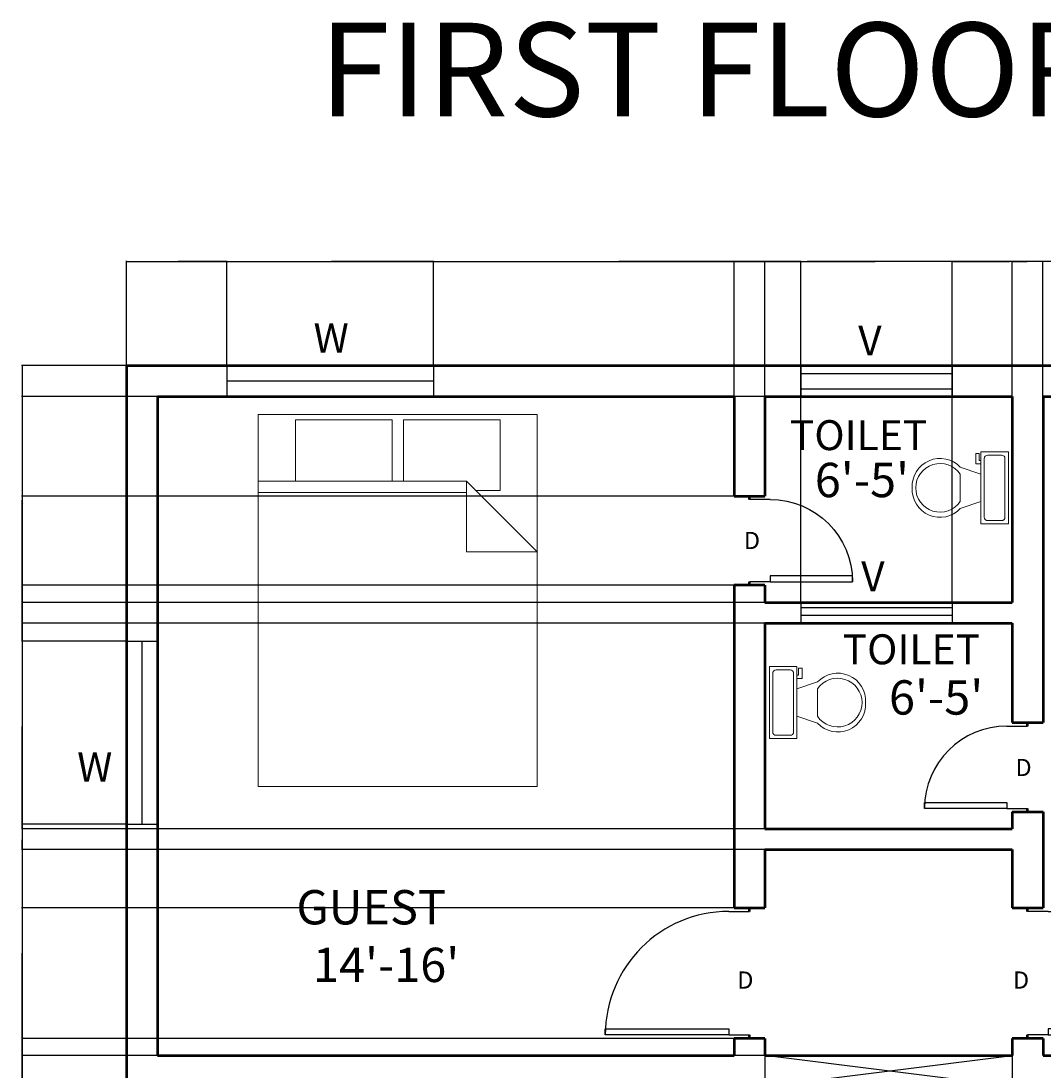
# Model space of a CAD drawing. Units: inches. Extents: x 2164 to 3752, y 2015 to 2629.
# Tile 7 of 8: x 3295 to 3592, y 2323 to 2629. Entities that reach past the tile are written whole.
import ezdxf
from ezdxf.enums import TextEntityAlignment as Align

# ---------------------------------------------------------------- set-up
doc = ezdxf.new("R2010")
doc.units = ezdxf.units.IN
for name, color, linetype, lineweight in [('A-ANNO-DIMS', 2, 'Continuous', 18), ('A-ANNO-TEXT', 7, 'Continuous', 25), ('A-AREA-IDEN', 3, 'Continuous', 25), ('A-DOOR', 3, 'Continuous', 25), ('A-FLOR-FIXT', 8, 'Continuous', 18), ('A-FURN', 8, 'Continuous', 18), ('A-GLAZ', 4, 'Continuous', 25), ('A-WALL', 7, 'Continuous', 50)]:
    doc.layers.add(name, color=color, linetype=linetype, lineweight=lineweight)
doc.styles.get("Standard").update_dxf_attribs({"font": 'arial.ttf'})
doc.dimstyles.get("Standard").update_dxf_attribs({"dimtxt": 0.18, "dimasz": 0.18, "dimexe": 0.18, "dimexo": 0.0625, "dimgap": 0.09, "dimtad": 0, "dimtih": 1, "dimtoh": 1, "dimdec": 4, "dimzin": 0, "dimdsep": 46, "dimtxsty": 'Standard', "dimcen": 0.09, "dimadec": 0, "dimazin": 0, "dimtfac": 1, "dimtdec": 4, "dimtofl": 0, "dimtmove": 0, "dimatfit": 3, "dimfxl": 1, "dimtolj": 1, "dimtzin": 0, "dimarcsym": 0})

# ---------------------------------------------------------------- blocks, each defined once
blk = doc.blocks.new('*U4')
for p, q in [((9.5, -6), (9.5, -2)), ((-10, -8.5), (-8, -8.5)), ((-10, -9.5), (-10, -8.5)), ((-8, -8.5), (-8, -8)), ((-7, -8), (-7, -9.5)), ((-4, -8), (-6, -14)), ((4, -8), (6, -14)), ((-7, -9.5), (-10, -9.5)), ((4, -14), (-4, -14))]:
    blk.add_line(p, q)
blk.add_lwpolyline([(10.5, -8), (10.5, 0), (-10.5, 0), (-10.5, -8)], close=True)
for points in [[(-9.5, -2), (-9.5, -6)], [(8.5, -1), (-8.5, -1)], [(-8.5, -7), (8.5, -7)]]:
    blk.add_lwpolyline(points)
for centre, radius, start, end in [((-8.625, -1.875), 0.8839, 81.8699, 188.1301), ((8.625, -1.875), 0.8839, 351.8699, 98.1301), ((-8.625, -6.125), 0.8839, 171.869898, 278.1301), ((8.625, -6.125), 0.8839, 261.8699, 8.1301), ((-0.4772, -19.9188), 8.0953, 133.01722, 273.38), ((0.0374, -19.8731), 7.127, 124.50543, 269.7), ((-0.0373, -19.8731), 7.127, 270.3, 55.4946), ((0.4773, -19.9188), 8.0953, 266.62, 46.9828)]:
    blk.add_arc(centre, radius, start, end)
blk = doc.blocks.new('*U2')
for p, q in [((0, 0), (0, -6)), ((24, 0), (24, -6))]:
    blk.add_line(p, q)
blk.add_lwpolyline([(0, 0), (0, 24), (1.75, 24), (1.75, 0)], close=True)
blk.add_arc((0, 0), 24, 0, 90)
blk = doc.blocks.new('*U6')
for p, q in [((0, 0), (0, -6)), ((36, 0), (36, -6))]:
    blk.add_line(p, q)
blk.add_lwpolyline([(0, 0), (0, 36), (1.75, 36), (1.75, 0)], close=True)
blk.add_arc((0, 0), 36, 0, 90)
blk = doc.blocks.new('Bed - Queen')
for p, q in [((0, -80.00003), (0, 0)), ((0, 0), (59.99999, 0)), ((59.99999, 0), (59.99999, -80.00003)), ((7.99999, -1.2), (28.79998, -1.2)), ((7.99999, -14.4), (7.99999, -1.2)), ((28.79998, -1.2), (28.79998, -14.4)), ((31.19999, -1.2), (51.99999, -1.2)), ((31.19999, -14.4), (31.19999, -1.2)), ((51.99999, -1.2), (51.99999, -16.4)), ((0, -14.4), (44.8, -14.4)), ((59.99999, -29.6), (44.8, -14.4)), ((44.8, -14.4), (44.8, -29.6)), ((44.8, -16.8), (0, -16.8)), ((51.99999, -16.4), (46.79936, -16.4)), ((44.8, -29.6), (59.99999, -29.6)), ((59.99999, -80.00003), (0, -80.00003))]:
    blk.add_line(p, q)
blk = doc.blocks.new('VENTILATOR')
for p, q in [((2394.78, 2528.72), (2394.78, 2519.72)), ((2438.92, 2528.72), (2438.92, 2519.72)), ((2394.78, 2526.43), (2438.92, 2526.43)), ((2438.92, 2521.87), (2394.78, 2521.87))]:
    blk.add_line(p, q)
blk = doc.blocks.new('*D99')
at = {"layer": 'A-ANNO-DIMS', "color": 0, "lineweight": -2, "transparency": 16777216}
for p, q in [((3325.39, 2528.78), (3325.39, 2559.25)), ((3325.57, 2559.07), (3339.56, 2559.07)), ((3354.47, 2559.07), (3340.49, 2559.07)), ((3354.65, 2528.78), (3354.65, 2559.25))]:
    blk.add_line(p, q, dxfattribs=at)
at = {"layer": 'A-ANNO-DIMS', "color": 0, "transparency": 16777216}
for points in [[(3325.57, 2559.1), (3325.57, 2559.04), (3325.39, 2559.07)], [(3354.47, 2559.1), (3354.47, 2559.04), (3354.65, 2559.07)]]:
    blk.add_solid(points, dxfattribs=at)
at = {"layer": 'Defpoints', "color": 0, "transparency": 16777216}
for p in [(3354.65, 2559.07), (3325.39, 2528.72), (3354.65, 2528.72)]:
    blk.add_point(p, dxfattribs=at)
at = {"layer": 'A-ANNO-DIMS', "color": 0, "transparency": 16777216, "insert": (3340.02, 2559.07), "char_height": 0.18, "attachment_point": 5}
blk.add_mtext('\\A1;29.254', dxfattribs=at)
blk = doc.blocks.new('*D100')
at = {"layer": 'A-ANNO-DIMS', "color": 0, "lineweight": -2, "transparency": 16777216}
for p, q in [((3354.65, 2528.78), (3354.65, 2559.25)), ((3354.83, 2559.07), (3384.36, 2559.07)), ((3414.69, 2559.07), (3385.15, 2559.07)), ((3414.87, 2528.78), (3414.87, 2559.25))]:
    blk.add_line(p, q, dxfattribs=at)
at = {"layer": 'A-ANNO-DIMS', "color": 0, "transparency": 16777216}
for points in [[(3354.83, 2559.1), (3354.83, 2559.04), (3354.65, 2559.07)], [(3414.69, 2559.1), (3414.69, 2559.04), (3414.87, 2559.07)]]:
    blk.add_solid(points, dxfattribs=at)
at = {"layer": 'Defpoints', "color": 0, "transparency": 16777216}
for p in [(3414.87, 2559.07), (3354.65, 2528.72), (3414.87, 2528.72)]:
    blk.add_point(p, dxfattribs=at)
at = {"layer": 'A-ANNO-DIMS', "color": 0, "transparency": 16777216, "insert": (3384.76, 2559.07), "char_height": 0.18, "attachment_point": 5}
blk.add_mtext('\\A1;60.22', dxfattribs=at)
blk = doc.blocks.new('*D101')
at = {"layer": 'A-ANNO-DIMS', "color": 0, "lineweight": -2, "transparency": 16777216}
for p, q in [((3414.87, 2528.78), (3414.87, 2559.25)), ((3415.05, 2559.07), (3467.9, 2559.07)), ((3521.66, 2559.07), (3468.81, 2559.07)), ((3521.84, 2528.78), (3521.84, 2559.25))]:
    blk.add_line(p, q, dxfattribs=at)
at = {"layer": 'A-ANNO-DIMS', "color": 0, "transparency": 16777216}
for points in [[(3415.05, 2559.1), (3415.05, 2559.04), (3414.87, 2559.07)], [(3521.66, 2559.1), (3521.66, 2559.04), (3521.84, 2559.07)]]:
    blk.add_solid(points, dxfattribs=at)
at = {"layer": 'Defpoints', "color": 0, "transparency": 16777216}
for p in [(3521.84, 2559.07), (3414.87, 2528.72), (3521.84, 2528.72)]:
    blk.add_point(p, dxfattribs=at)
at = {"layer": 'A-ANNO-DIMS', "color": 0, "transparency": 16777216, "insert": (3468.35, 2559.07), "char_height": 0.18, "attachment_point": 5}
blk.add_mtext('\\A1;106.97', dxfattribs=at)
blk = doc.blocks.new('*D102')
at = {"layer": 'A-ANNO-DIMS', "color": 0, "lineweight": -2, "transparency": 16777216}
for p, q in [((3521.84, 2528.78), (3521.84, 2559.25)), ((3522.02, 2559.07), (3543.5, 2559.07)), ((3565.79, 2559.07), (3544.3, 2559.07)), ((3565.97, 2528.78), (3565.97, 2559.25))]:
    blk.add_line(p, q, dxfattribs=at)
at = {"layer": 'A-ANNO-DIMS', "color": 0, "transparency": 16777216}
for points in [[(3522.02, 2559.1), (3522.02, 2559.04), (3521.84, 2559.07)], [(3565.79, 2559.1), (3565.79, 2559.04), (3565.97, 2559.07)]]:
    blk.add_solid(points, dxfattribs=at)
at = {"layer": 'Defpoints', "color": 0, "transparency": 16777216}
for p in [(3565.97, 2559.07), (3521.84, 2528.72), (3565.97, 2528.72)]:
    blk.add_point(p, dxfattribs=at)
at = {"layer": 'A-ANNO-DIMS', "color": 0, "transparency": 16777216, "insert": (3543.9, 2559.07), "char_height": 0.18, "attachment_point": 5}
blk.add_mtext('\\A1;44.13', dxfattribs=at)
blk = doc.blocks.new('*D103')
at = {"layer": 'A-ANNO-DIMS', "color": 0, "lineweight": -2, "transparency": 16777216}
for p, q in [((3565.97, 2528.78), (3565.97, 2559.25)), ((3566.15, 2559.07), (3582.66, 2559.07)), ((3599.96, 2559.07), (3583.45, 2559.07)), ((3600.14, 2528.78), (3600.14, 2559.25))]:
    blk.add_line(p, q, dxfattribs=at)
at = {"layer": 'A-ANNO-DIMS', "color": 0, "transparency": 16777216}
for points in [[(3566.15, 2559.1), (3566.15, 2559.04), (3565.97, 2559.07)], [(3599.96, 2559.1), (3599.96, 2559.04), (3600.14, 2559.07)]]:
    blk.add_solid(points, dxfattribs=at)
at = {"layer": 'Defpoints', "color": 0, "transparency": 16777216}
for p in [(3600.14, 2559.07), (3565.97, 2528.72), (3600.14, 2528.72)]:
    blk.add_point(p, dxfattribs=at)
at = {"layer": 'A-ANNO-DIMS', "color": 0, "transparency": 16777216, "insert": (3583.05, 2559.07), "char_height": 0.18, "attachment_point": 5}
blk.add_mtext('\\A1;34.17', dxfattribs=at)
blk = doc.blocks.new('*D106')
at = {"layer": 'A-ANNO-DIMS', "color": 0, "lineweight": -2, "transparency": 16777216}
for p, q in [((3325.39, 2528.78), (3325.39, 2559.25)), ((3325.57, 2559.07), (3523.11, 2559.07)), ((3721.21, 2559.07), (3523.68, 2559.07)), ((3721.39, 2528.78), (3721.39, 2559.25))]:
    blk.add_line(p, q, dxfattribs=at)
at = {"layer": 'A-ANNO-DIMS', "color": 0, "transparency": 16777216}
for points in [[(3325.57, 2559.1), (3325.57, 2559.04), (3325.39, 2559.07)], [(3721.21, 2559.1), (3721.21, 2559.04), (3721.39, 2559.07)]]:
    blk.add_solid(points, dxfattribs=at)
at = {"layer": 'Defpoints', "color": 0, "transparency": 16777216}
for p in [(3721.39, 2559.07), (3325.39, 2528.72), (3721.39, 2528.72)]:
    blk.add_point(p, dxfattribs=at)
at = {"layer": 'A-ANNO-DIMS', "color": 0, "transparency": 16777216, "insert": (3523.39, 2559.07), "char_height": 0.18, "attachment_point": 5}
blk.add_mtext('\\A1;396', dxfattribs=at)
blk = doc.blocks.new('*D107')
at = {"layer": 'A-ANNO-DIMS', "color": 0, "lineweight": -2, "transparency": 16777216}
for p, q in [((3502.39, 2519.78), (3502.39, 2559.25)), ((3502.57, 2559.07), (3506.75, 2559.07)), ((3511.21, 2559.07), (3507.04, 2559.07)), ((3511.39, 2519.78), (3511.39, 2559.25))]:
    blk.add_line(p, q, dxfattribs=at)
at = {"layer": 'A-ANNO-DIMS', "color": 0, "transparency": 16777216}
for points in [[(3502.57, 2559.1), (3502.57, 2559.04), (3502.39, 2559.07)], [(3511.21, 2559.1), (3511.21, 2559.04), (3511.39, 2559.07)]]:
    blk.add_solid(points, dxfattribs=at)
at = {"layer": 'Defpoints', "color": 0, "transparency": 16777216}
for p in [(3511.39, 2559.07), (3502.39, 2519.72), (3511.39, 2519.72)]:
    blk.add_point(p, dxfattribs=at)
at = {"layer": 'A-ANNO-DIMS', "color": 0, "transparency": 16777216, "insert": (3506.89, 2559.07), "char_height": 0.18, "attachment_point": 5}
blk.add_mtext('\\A1;9', dxfattribs=at)
blk = doc.blocks.new('*D108')
at = {"layer": 'A-ANNO-DIMS', "color": 0, "lineweight": -2, "transparency": 16777216}
for p, q in [((3511.39, 2519.78), (3511.39, 2559.25)), ((3511.57, 2559.07), (3516.23, 2559.07)), ((3521.66, 2559.07), (3517, 2559.07)), ((3521.84, 2519.78), (3521.84, 2559.25))]:
    blk.add_line(p, q, dxfattribs=at)
at = {"layer": 'A-ANNO-DIMS', "color": 0, "transparency": 16777216}
for points in [[(3511.57, 2559.1), (3511.57, 2559.04), (3511.39, 2559.07)], [(3521.66, 2559.1), (3521.66, 2559.04), (3521.84, 2559.07)]]:
    blk.add_solid(points, dxfattribs=at)
at = {"layer": 'Defpoints', "color": 0, "transparency": 16777216}
for p in [(3521.84, 2559.07), (3511.39, 2519.72), (3521.84, 2519.72)]:
    blk.add_point(p, dxfattribs=at)
at = {"layer": 'A-ANNO-DIMS', "color": 0, "transparency": 16777216, "insert": (3516.62, 2559.07), "char_height": 0.18, "attachment_point": 5}
blk.add_mtext('\\A1;10.44', dxfattribs=at)
blk = doc.blocks.new('*D109')
at = {"layer": 'A-ANNO-DIMS', "color": 0, "lineweight": -2, "transparency": 16777216}
for p, q in [((3565.97, 2519.78), (3565.97, 2559.25)), ((3566.15, 2559.07), (3574.23, 2559.07)), ((3583.21, 2559.07), (3575.14, 2559.07)), ((3583.39, 2519.78), (3583.39, 2559.25))]:
    blk.add_line(p, q, dxfattribs=at)
at = {"layer": 'A-ANNO-DIMS', "color": 0, "transparency": 16777216}
for points in [[(3566.15, 2559.1), (3566.15, 2559.04), (3565.97, 2559.07)], [(3583.21, 2559.1), (3583.21, 2559.04), (3583.39, 2559.07)]]:
    blk.add_solid(points, dxfattribs=at)
at = {"layer": 'Defpoints', "color": 0, "transparency": 16777216}
for p in [(3583.39, 2559.07), (3565.97, 2519.72), (3583.39, 2519.72)]:
    blk.add_point(p, dxfattribs=at)
at = {"layer": 'A-ANNO-DIMS', "color": 0, "transparency": 16777216, "insert": (3574.68, 2559.07), "char_height": 0.18, "attachment_point": 5}
blk.add_mtext('\\A1;17.426', dxfattribs=at)
blk = doc.blocks.new('*D110')
at = {"layer": 'A-ANNO-DIMS', "color": 0, "lineweight": -2, "transparency": 16777216}
for p, q in [((3583.39, 2519.78), (3583.39, 2559.25)), ((3583.57, 2559.07), (3587.75, 2559.07)), ((3592.21, 2559.07), (3588.04, 2559.07)), ((3592.39, 2519.78), (3592.39, 2559.25))]:
    blk.add_line(p, q, dxfattribs=at)
at = {"layer": 'A-ANNO-DIMS', "color": 0, "transparency": 16777216}
for points in [[(3583.57, 2559.1), (3583.57, 2559.04), (3583.39, 2559.07)], [(3592.21, 2559.1), (3592.21, 2559.04), (3592.39, 2559.07)]]:
    blk.add_solid(points, dxfattribs=at)
at = {"layer": 'Defpoints', "color": 0, "transparency": 16777216}
for p in [(3592.39, 2559.07), (3583.39, 2519.72), (3592.39, 2519.72)]:
    blk.add_point(p, dxfattribs=at)
at = {"layer": 'A-ANNO-DIMS', "color": 0, "transparency": 16777216, "insert": (3587.89, 2559.07), "char_height": 0.18, "attachment_point": 5}
blk.add_mtext('\\A1;9', dxfattribs=at)
blk = doc.blocks.new('*D124')
at = {"layer": 'A-ANNO-DIMS', "color": 0, "lineweight": -2, "transparency": 16777216}
for p, q in [((3325.33, 2395.15), (3294.86, 2395.15)), ((3295.04, 2394.97), (3295.04, 2337.1)), ((3295.04, 2278.87), (3295.04, 2336.74)), ((3325.33, 2278.69), (3294.86, 2278.69))]:
    blk.add_line(p, q, dxfattribs=at)
at = {"layer": 'A-ANNO-DIMS', "color": 0, "transparency": 16777216}
for points in [[(3295.01, 2394.97), (3295.07, 2394.97), (3295.04, 2395.15)], [(3295.01, 2278.87), (3295.07, 2278.87), (3295.04, 2278.69)]]:
    blk.add_solid(points, dxfattribs=at)
at = {"layer": 'Defpoints', "color": 0, "transparency": 16777216}
for p in [(3295.04, 2395.15), (3325.39, 2395.15), (3325.39, 2278.69)]:
    blk.add_point(p, dxfattribs=at)
at = {"layer": 'A-ANNO-DIMS', "color": 0, "transparency": 16777216, "insert": (3295.04, 2336.92), "char_height": 0.18, "attachment_point": 5}
blk.add_mtext('\\A1;116.47', dxfattribs=at)
blk = doc.blocks.new('*D125')
at = {"layer": 'A-ANNO-DIMS', "color": 0, "lineweight": -2, "transparency": 16777216}
for p, q in [((3325.33, 2448.4), (3294.86, 2448.4)), ((3295.04, 2448.22), (3295.04, 2421.96)), ((3295.04, 2395.33), (3295.04, 2421.59)), ((3325.33, 2395.15), (3294.86, 2395.15))]:
    blk.add_line(p, q, dxfattribs=at)
at = {"layer": 'A-ANNO-DIMS', "color": 0, "transparency": 16777216}
for points in [[(3295.01, 2448.22), (3295.07, 2448.22), (3295.04, 2448.4)], [(3295.01, 2395.33), (3295.07, 2395.33), (3295.04, 2395.15)]]:
    blk.add_solid(points, dxfattribs=at)
at = {"layer": 'Defpoints', "color": 0, "transparency": 16777216}
for p in [(3295.04, 2448.4), (3325.39, 2448.4), (3325.39, 2395.15)]:
    blk.add_point(p, dxfattribs=at)
at = {"layer": 'A-ANNO-DIMS', "color": 0, "transparency": 16777216, "insert": (3295.04, 2421.78), "char_height": 0.18, "attachment_point": 5}
blk.add_mtext('\\A1;53.25', dxfattribs=at)
blk = doc.blocks.new('*D126')
at = {"layer": 'A-ANNO-DIMS', "color": 0, "lineweight": -2, "transparency": 16777216}
for p, q in [((3325.33, 2528.72), (3294.86, 2528.72)), ((3295.04, 2528.54), (3295.04, 2488.74)), ((3295.04, 2448.58), (3295.04, 2488.38)), ((3325.33, 2448.4), (3294.86, 2448.4))]:
    blk.add_line(p, q, dxfattribs=at)
at = {"layer": 'A-ANNO-DIMS', "color": 0, "transparency": 16777216}
for points in [[(3295.01, 2528.54), (3295.07, 2528.54), (3295.04, 2528.72)], [(3295.01, 2448.58), (3295.07, 2448.58), (3295.04, 2448.4)]]:
    blk.add_solid(points, dxfattribs=at)
at = {"layer": 'Defpoints', "color": 0, "transparency": 16777216}
for p in [(3295.04, 2528.72), (3325.39, 2528.72), (3325.39, 2448.4)]:
    blk.add_point(p, dxfattribs=at)
at = {"layer": 'A-ANNO-DIMS', "color": 0, "transparency": 16777216, "insert": (3295.04, 2488.56), "char_height": 0.18, "attachment_point": 5}
blk.add_mtext('\\A1;80.32', dxfattribs=at)
blk = doc.blocks.new('*D127')
at = {"layer": 'A-ANNO-DIMS', "color": 0, "lineweight": -2, "transparency": 16777216}
for p, q in [((3325.33, 2528.72), (3294.86, 2528.72)), ((3295.04, 2528.54), (3295.04, 2287.4)), ((3295.04, 2045.9), (3295.04, 2287.04)), ((3325.33, 2045.72), (3294.86, 2045.72))]:
    blk.add_line(p, q, dxfattribs=at)
at = {"layer": 'A-ANNO-DIMS', "color": 0, "transparency": 16777216}
for points in [[(3295.01, 2528.54), (3295.07, 2528.54), (3295.04, 2528.72)], [(3295.01, 2045.9), (3295.07, 2045.9), (3295.04, 2045.72)]]:
    blk.add_solid(points, dxfattribs=at)
at = {"layer": 'Defpoints', "color": 0, "transparency": 16777216}
for p in [(3295.04, 2528.72), (3325.39, 2528.72), (3325.39, 2045.72)]:
    blk.add_point(p, dxfattribs=at)
at = {"layer": 'A-ANNO-DIMS', "color": 0, "transparency": 16777216, "insert": (3295.04, 2287.22), "char_height": 0.18, "attachment_point": 5}
blk.add_mtext('\\A1;483', dxfattribs=at)
blk = doc.blocks.new('*D139')
at = {"layer": 'A-ANNO-DIMS', "color": 0, "lineweight": -2, "transparency": 16777216}
for p, q in [((3511.33, 2387.72), (3294.86, 2387.72)), ((3295.04, 2387.54), (3295.04, 2357.9)), ((3295.04, 2327.9), (3295.04, 2357.54)), ((3511.33, 2327.72), (3294.86, 2327.72))]:
    blk.add_line(p, q, dxfattribs=at)
at = {"layer": 'A-ANNO-DIMS', "color": 0, "transparency": 16777216}
for points in [[(3295.01, 2387.54), (3295.07, 2387.54), (3295.04, 2387.72)], [(3295.01, 2327.9), (3295.07, 2327.9), (3295.04, 2327.72)]]:
    blk.add_solid(points, dxfattribs=at)
at = {"layer": 'Defpoints', "color": 0, "transparency": 16777216}
for p in [(3295.04, 2387.72), (3511.39, 2387.72), (3511.39, 2327.72)]:
    blk.add_point(p, dxfattribs=at)
at = {"layer": 'A-ANNO-DIMS', "color": 0, "transparency": 16777216, "insert": (3295.04, 2357.72), "char_height": 0.18, "attachment_point": 5}
blk.add_mtext('\\A1;60', dxfattribs=at)
blk = doc.blocks.new('*D140')
at = {"layer": 'A-ANNO-DIMS', "color": 0, "lineweight": -2, "transparency": 16777216}
for p, q in [((3511.33, 2393.72), (3294.86, 2393.72)), ((3295.04, 2393.54), (3295.04, 2390.9)), ((3295.04, 2387.9), (3295.04, 2390.54)), ((3511.33, 2387.72), (3294.86, 2387.72))]:
    blk.add_line(p, q, dxfattribs=at)
at = {"layer": 'A-ANNO-DIMS', "color": 0, "transparency": 16777216}
for points in [[(3295.01, 2393.54), (3295.07, 2393.54), (3295.04, 2393.72)], [(3295.01, 2387.9), (3295.07, 2387.9), (3295.04, 2387.72)]]:
    blk.add_solid(points, dxfattribs=at)
at = {"layer": 'Defpoints', "color": 0, "transparency": 16777216}
for p in [(3295.04, 2393.72), (3511.39, 2393.72), (3511.39, 2387.72)]:
    blk.add_point(p, dxfattribs=at)
at = {"layer": 'A-ANNO-DIMS', "color": 0, "transparency": 16777216, "insert": (3295.04, 2390.72), "char_height": 0.18, "attachment_point": 5}
blk.add_mtext('\\A1;6', dxfattribs=at)
blk = doc.blocks.new('*D141')
at = {"layer": 'A-ANNO-DIMS', "color": 0, "lineweight": -2, "transparency": 16777216}
for p, q in [((3511.33, 2453.72), (3294.86, 2453.72)), ((3295.04, 2453.54), (3295.04, 2423.9)), ((3295.04, 2393.9), (3295.04, 2423.54)), ((3511.33, 2393.72), (3294.86, 2393.72))]:
    blk.add_line(p, q, dxfattribs=at)
at = {"layer": 'A-ANNO-DIMS', "color": 0, "transparency": 16777216}
for points in [[(3295.01, 2453.54), (3295.07, 2453.54), (3295.04, 2453.72)], [(3295.01, 2393.9), (3295.07, 2393.9), (3295.04, 2393.72)]]:
    blk.add_solid(points, dxfattribs=at)
at = {"layer": 'Defpoints', "color": 0, "transparency": 16777216}
for p in [(3295.04, 2453.72), (3511.39, 2453.72), (3511.39, 2393.72)]:
    blk.add_point(p, dxfattribs=at)
at = {"layer": 'A-ANNO-DIMS', "color": 0, "transparency": 16777216, "insert": (3295.04, 2423.72), "char_height": 0.18, "attachment_point": 5}
blk.add_mtext('\\A1;60', dxfattribs=at)
blk = doc.blocks.new('*D142')
at = {"layer": 'A-ANNO-DIMS', "color": 0, "lineweight": -2, "transparency": 16777216}
for p, q in [((3511.33, 2459.72), (3294.86, 2459.72)), ((3295.04, 2459.54), (3295.04, 2456.9)), ((3295.04, 2453.9), (3295.04, 2456.54)), ((3511.33, 2453.72), (3294.86, 2453.72))]:
    blk.add_line(p, q, dxfattribs=at)
at = {"layer": 'A-ANNO-DIMS', "color": 0, "transparency": 16777216}
for points in [[(3295.01, 2459.54), (3295.07, 2459.54), (3295.04, 2459.72)], [(3295.01, 2453.9), (3295.07, 2453.9), (3295.04, 2453.72)]]:
    blk.add_solid(points, dxfattribs=at)
at = {"layer": 'Defpoints', "color": 0, "transparency": 16777216}
for p in [(3295.04, 2459.72), (3511.39, 2459.72), (3511.39, 2453.72)]:
    blk.add_point(p, dxfattribs=at)
at = {"layer": 'A-ANNO-DIMS', "color": 0, "transparency": 16777216, "insert": (3295.04, 2456.72), "char_height": 0.18, "attachment_point": 5}
blk.add_mtext('\\A1;6', dxfattribs=at)
blk = doc.blocks.new('*D143')
at = {"layer": 'A-ANNO-DIMS', "color": 0, "lineweight": -2, "transparency": 16777216}
for p, q in [((3511.33, 2519.72), (3294.86, 2519.72)), ((3295.04, 2519.54), (3295.04, 2489.9)), ((3295.04, 2459.9), (3295.04, 2489.54)), ((3511.33, 2459.72), (3294.86, 2459.72))]:
    blk.add_line(p, q, dxfattribs=at)
at = {"layer": 'A-ANNO-DIMS', "color": 0, "transparency": 16777216}
for points in [[(3295.01, 2519.54), (3295.07, 2519.54), (3295.04, 2519.72)], [(3295.01, 2459.9), (3295.07, 2459.9), (3295.04, 2459.72)]]:
    blk.add_solid(points, dxfattribs=at)
at = {"layer": 'Defpoints', "color": 0, "transparency": 16777216}
for p in [(3295.04, 2519.72), (3511.39, 2519.72), (3511.39, 2459.72)]:
    blk.add_point(p, dxfattribs=at)
at = {"layer": 'A-ANNO-DIMS', "color": 0, "transparency": 16777216, "insert": (3295.04, 2489.72), "char_height": 0.18, "attachment_point": 5}
blk.add_mtext('\\A1;60', dxfattribs=at)
blk = doc.blocks.new('*D144')
at = {"layer": 'A-ANNO-DIMS', "color": 0, "lineweight": -2, "transparency": 16777216}
for p, q in [((3502.33, 2490.72), (3294.86, 2490.72)), ((3295.04, 2490.54), (3295.04, 2477.9)), ((3295.04, 2464.9), (3295.04, 2477.54)), ((3502.33, 2464.72), (3294.86, 2464.72))]:
    blk.add_line(p, q, dxfattribs=at)
at = {"layer": 'A-ANNO-DIMS', "color": 0, "transparency": 16777216}
for points in [[(3295.01, 2490.54), (3295.07, 2490.54), (3295.04, 2490.72)], [(3295.01, 2464.9), (3295.07, 2464.9), (3295.04, 2464.72)]]:
    blk.add_solid(points, dxfattribs=at)
at = {"layer": 'Defpoints', "color": 0, "transparency": 16777216}
for p in [(3295.04, 2490.72), (3502.39, 2490.72), (3502.39, 2464.72)]:
    blk.add_point(p, dxfattribs=at)
at = {"layer": 'A-ANNO-DIMS', "color": 0, "transparency": 16777216, "insert": (3295.04, 2477.72), "char_height": 0.18, "attachment_point": 5}
blk.add_mtext('\\A1;26', dxfattribs=at)
blk = doc.blocks.new('*D146')
at = {"layer": 'A-ANNO-DIMS', "color": 0, "lineweight": -2, "transparency": 16777216}
for p, q in [((3502.33, 2370.72), (3294.86, 2370.72)), ((3295.04, 2370.54), (3295.04, 2351.9)), ((3295.04, 2332.9), (3295.04, 2351.54)), ((3502.33, 2332.72), (3294.86, 2332.72))]:
    blk.add_line(p, q, dxfattribs=at)
at = {"layer": 'A-ANNO-DIMS', "color": 0, "transparency": 16777216}
for points in [[(3295.01, 2370.54), (3295.07, 2370.54), (3295.04, 2370.72)], [(3295.01, 2332.9), (3295.07, 2332.9), (3295.04, 2332.72)]]:
    blk.add_solid(points, dxfattribs=at)
at = {"layer": 'Defpoints', "color": 0, "transparency": 16777216}
for p in [(3295.04, 2370.72), (3502.39, 2370.72), (3502.39, 2332.72)]:
    blk.add_point(p, dxfattribs=at)
at = {"layer": 'A-ANNO-DIMS', "color": 0, "transparency": 16777216, "insert": (3295.04, 2351.72), "char_height": 0.18, "attachment_point": 5}
blk.add_mtext('\\A1;38', dxfattribs=at)
blk = doc.blocks.new('*D149')
at = {"layer": 'A-ANNO-DIMS', "color": 0, "lineweight": -2, "transparency": 16777216}
for p, q in [((3521.84, 2459.78), (3521.84, 2559.25)), ((3522.02, 2559.07), (3543.5, 2559.07)), ((3565.79, 2559.07), (3544.3, 2559.07)), ((3565.97, 2459.78), (3565.97, 2559.25))]:
    blk.add_line(p, q, dxfattribs=at)
at = {"layer": 'A-ANNO-DIMS', "color": 0, "transparency": 16777216}
for points in [[(3522.02, 2559.1), (3522.02, 2559.04), (3521.84, 2559.07)], [(3565.79, 2559.1), (3565.79, 2559.04), (3565.97, 2559.07)]]:
    blk.add_solid(points, dxfattribs=at)
at = {"layer": 'Defpoints', "color": 0, "transparency": 16777216}
for p in [(3565.97, 2559.07), (3521.84, 2459.72), (3565.97, 2459.72)]:
    blk.add_point(p, dxfattribs=at)
at = {"layer": 'A-ANNO-DIMS', "color": 0, "transparency": 16777216, "insert": (3543.9, 2559.07), "char_height": 0.18, "attachment_point": 5}
blk.add_mtext('\\A1;44.13', dxfattribs=at)

msp = doc.modelspace()

# ---------------------------------------------------------------- linework, layer by layer
at = {"layer": 'A-GLAZ'}
for p, q in [((3354.6488, 2528.7172), (3354.6488, 2519.7172)), ((3414.8658, 2528.7172), (3414.8658, 2519.7172)), ((3414.8658, 2524.2172), (3354.6488, 2524.2172)), ((3521.8355, 2459.7172), (3521.8355, 2453.7172)), ((3565.9689, 2459.7172), (3565.9689, 2453.7172)), ((3521.8355, 2458.2172), (3565.9689, 2458.2172)), ((3565.9689, 2455.8656), (3521.8355, 2455.8656)), ((3325.395, 2448.3998), (3334.395, 2448.3998)), ((3329.895, 2448.3998), (3329.895, 2395.1516)), ((3325.395, 2395.1516), (3334.395, 2395.1516)), ((3511.395, 2327.7172), (3511.395, 2318.7172)), ((3511.395, 2318.7172), (3583.395, 2327.7172)), ((3583.395, 2318.7172), (3511.395, 2327.7172)), ((3583.395, 2327.7172), (3583.395, 2318.7172))]:
    msp.add_line(p, q, dxfattribs=at)
at = {"layer": 'A-WALL'}
for p, q in [((3325.395, 2528.7172), (3721.395, 2528.7172)), ((3325.395, 2528.7172), (3325.395, 2045.7172)), ((3334.395, 2519.7172), (3334.395, 2327.7172)), ((3334.395, 2519.7172), (3502.395, 2519.7172)), ((3502.395, 2519.7172), (3502.395, 2490.7172)), ((3511.395, 2519.7172), (3511.395, 2490.7172)), ((3511.395, 2519.7172), (3583.395, 2519.7172)), ((3583.395, 2519.7172), (3583.395, 2459.7172)), ((3592.395, 2519.7172), (3592.395, 2424.7172)), ((3592.395, 2519.7172), (3712.395, 2519.7172)), ((3502.395, 2490.7172), (3511.395, 2490.7172)), ((3506.895, 2489.7172), (3506.895, 2490.7172)), ((3506.895, 2464.7172), (3506.895, 2465.7172)), ((3511.395, 2464.7172), (3502.395, 2464.7172)), ((3502.395, 2464.7172), (3502.395, 2370.7172)), ((3511.395, 2464.7172), (3511.395, 2459.7172)), ((3511.395, 2459.7172), (3583.395, 2459.7172)), ((3511.395, 2453.7172), (3583.395, 2453.7172)), ((3511.395, 2453.7172), (3511.395, 2393.7172)), ((3583.395, 2453.7172), (3583.395, 2424.7172)), ((3583.395, 2424.7172), (3592.395, 2424.7172)), ((3587.895, 2423.7172), (3587.895, 2424.7172)), ((3583.395, 2398.7172), (3592.395, 2398.7172)), ((3583.395, 2398.7172), (3583.395, 2393.7172)), ((3587.895, 2398.7172), (3587.895, 2399.7172)), ((3592.395, 2398.7172), (3592.395, 2370.7172)), ((3511.395, 2393.7172), (3583.395, 2393.7172)), ((3511.395, 2387.7172), (3583.395, 2387.7172)), ((3511.395, 2387.7172), (3511.395, 2370.7172)), ((3583.395, 2387.7172), (3583.395, 2370.7172)), ((3502.395, 2370.7172), (3511.395, 2370.7172)), ((3506.895, 2369.7172), (3506.895, 2370.7172)), ((3583.395, 2370.7172), (3592.395, 2370.7172)), ((3587.895, 2369.7172), (3587.895, 2370.7172)), ((3511.395, 2332.7172), (3502.395, 2332.7172)), ((3502.395, 2332.7172), (3502.395, 2327.7172)), ((3506.895, 2332.7172), (3506.895, 2333.7172)), ((3511.395, 2332.7172), (3511.395, 2327.7172)), ((3592.395, 2332.7172), (3583.395, 2332.7172)), ((3583.395, 2332.7172), (3583.395, 2327.7172)), ((3587.895, 2332.7172), (3587.895, 2333.7172)), ((3592.395, 2332.7172), (3592.395, 2327.7172)), ((3334.395, 2327.7172), (3502.395, 2327.7172)), ((3511.395, 2327.7172), (3583.395, 2327.7172)), ((3592.395, 2327.7172), (3712.395, 2327.7172))]:
    msp.add_line(p, q, dxfattribs=at)

# ---------------------------------------------------------------- block references
at = {"layer": 'A-DOOR', "xscale": -1, "rotation": 270}
for name, p in [('*U2', (3512.895, 2465.7172)), ('*U6', (3593.895, 2333.7172))]:
    msp.add_blockref(name, p, dxfattribs=at)
at = {"layer": 'A-DOOR', "rotation": 90.00000000000003}
for name, p in [('*U2', (3581.895, 2399.7172)), ('*U6', (3500.895, 2333.7172))]:
    msp.add_blockref(name, p, dxfattribs=at)
at = {"layer": 'A-FLOR-FIXT', "rotation": 270}
msp.add_blockref('*U4', (3582.302, 2493.0967), dxfattribs=at)
at = {"layer": 'A-FLOR-FIXT', "xscale": -1, "rotation": 90}
msp.add_blockref('*U4', (3512.7007, 2430.5397), dxfattribs=at)
at = {"layer": 'A-FURN', "xscale": 1.354750275868299, "yscale": 1.354750275868299, "zscale": 1.354750275868299}
msp.add_blockref('Bed - Queen', (3363.7819, 2514.5121), dxfattribs=at)
at = {"layer": 'A-GLAZ'}
msp.add_blockref('VENTILATOR', (1127.0534, 0), dxfattribs=at)

# ---------------------------------------------------------------- texts
at = {"layer": 'A-ANNO-TEXT'}
for s, height, p in [('FIRST FLOOR', 27.32215, (3495.4066, 2611.4091)), ('W', 8.5558, (3385.0292, 2535.6454)), ('V', 8.7141, (3541.9633, 2534.8989)), ('V', 8.7141, (3542.8335, 2466.2099)), ('W', 8.5558, (3316.154, 2410.7032))]:
    msp.add_text(s, height=height, dxfattribs=at).set_placement(p, align=Align.MIDDLE)
for p in [(3505.2645, 2475.2663), (3584.3854, 2409.1274), (3503.3391, 2347.2146), (3583.6551, 2347.2146)]:
    msp.add_text('D', height=5, dxfattribs=at).set_placement(p)
at = {"layer": 'A-AREA-IDEN'}
for s, height, p in [('TOILET', 8.72285, (3518.6515, 2504.0893)), ("6'-5'", 10, (3525.9189, 2490.389)), ('TOILET', 8.72285, (3534.0212, 2441.7013)), ("6'-5'", 10, (3547.5326, 2427.0412)), ('GUEST', 10, (3374.9021, 2365.9204)), ("14'-16'", 10, (3379.738, 2349.1311))]:
    msp.add_text(s, height=height, dxfattribs=at).set_placement(p)

# ---------------------------------------------------------------- dimensions: what is measured, and where the dimension line sits
at = {"layer": 'A-ANNO-DIMS'}
for base, p1, p2, override, picture, middle in [((3354.6488, 2559.0672), (3325.395, 2528.7172), (3354.6488, 2528.7172), {"dimdec": 3, "dimlfac": 1, "dimrnd": 0, "dimzin": 0, "dimdsep": 46, "dimlunit": 2}, '*D99', (3340.0219, 2559.0672)), ((3721.395, 2559.0672), (3325.395, 2528.7172), (3721.395, 2528.7172), {"dimdec": 0, "dimlfac": 1, "dimrnd": 0, "dimzin": 0, "dimdsep": 46, "dimlunit": 2}, '*D106', (3523.395, 2559.0672)), ((3414.8658, 2559.0672), (3354.6488, 2528.7172), (3414.8658, 2528.7172), {"dimdec": 2, "dimlfac": 1, "dimrnd": 0, "dimzin": 0, "dimdsep": 46, "dimlunit": 2}, '*D100', (3384.7573, 2559.0672)), ((3521.8355, 2559.0672), (3414.8658, 2528.7172), (3521.8355, 2528.7172), {"dimdec": 2, "dimlfac": 1, "dimrnd": 0, "dimzin": 0, "dimdsep": 46, "dimlunit": 2}, '*D101', (3468.3506, 2559.0672)), ((3511.395, 2559.0672), (3502.395, 2519.7172), (3511.395, 2519.7172), {"dimdec": 0, "dimlfac": 1, "dimrnd": 0, "dimzin": 0, "dimdsep": 46, "dimlunit": 2}, '*D107', (3506.895, 2559.0672)), ((3521.8355, 2559.0672), (3511.395, 2519.7172), (3521.8355, 2519.7172), {"dimdec": 2, "dimlfac": 1, "dimrnd": 0, "dimzin": 0, "dimdsep": 46, "dimlunit": 2}, '*D108', (3516.6152, 2559.0672)), ((3565.9689, 2559.0672), (3521.8355, 2528.7172), (3565.9689, 2528.7172), {"dimdec": 2, "dimlfac": 1, "dimrnd": 0, "dimzin": 0, "dimdsep": 46, "dimlunit": 2}, '*D102', (3543.9022, 2559.0672)), ((3565.9689, 2559.0672), (3521.8355, 2459.7172), (3565.9689, 2459.7172), {"dimdec": 2, "dimlfac": 1, "dimrnd": 0, "dimzin": 0, "dimdsep": 46, "dimlunit": 2}, '*D149', (3543.9022, 2559.0672)), ((3600.1393, 2559.0672), (3565.9689, 2528.7172), (3600.1393, 2528.7172), {"dimdec": 2, "dimlfac": 1, "dimrnd": 0, "dimzin": 0, "dimdsep": 46, "dimlunit": 2}, '*D103', (3583.0541, 2559.0672)), ((3583.395, 2559.0672), (3565.9689, 2519.7172), (3583.395, 2519.7172), {"dimdec": 3, "dimlfac": 1, "dimrnd": 0, "dimzin": 0, "dimdsep": 46, "dimlunit": 2}, '*D109', (3574.6819, 2559.0672)), ((3592.395, 2559.0672), (3583.395, 2519.7172), (3592.395, 2519.7172), {"dimdec": 0, "dimlfac": 1, "dimrnd": 0, "dimzin": 0, "dimdsep": 46, "dimlunit": 2}, '*D110', (3587.895, 2559.0672))]:
    dim = msp.add_linear_dim(base=base, p1=p1, p2=p2, dimstyle='Standard', override=override, dxfattribs=at)
    dim.commit()
    dim.dimension.update_dxf_attribs({"geometry": picture, "text_midpoint": middle})
for base, p1, p2, override, picture, middle in [((3295.045, 2528.7172), (3325.395, 2448.3998), (3325.395, 2528.7172), {"dimdec": 2, "dimlfac": 1, "dimrnd": 0, "dimzin": 0, "dimdsep": 46, "dimlunit": 2}, '*D126', (3295.045, 2488.5585)), ((3295.045, 2528.7172), (3325.395, 2045.7172), (3325.395, 2528.7172), {"dimdec": 0, "dimlfac": 1, "dimrnd": 0, "dimzin": 0, "dimdsep": 46, "dimlunit": 2}, '*D127', (3295.045, 2287.2172)), ((3295.045, 2519.7172), (3511.395, 2459.7172), (3511.395, 2519.7172), {"dimdec": 0, "dimlfac": 1, "dimrnd": 0, "dimzin": 0, "dimdsep": 46, "dimlunit": 2}, '*D143', (3295.045, 2489.7172)), ((3295.045, 2490.7172), (3502.395, 2464.7172), (3502.395, 2490.7172), {"dimdec": 0, "dimlfac": 1, "dimrnd": 0, "dimzin": 0, "dimdsep": 46, "dimlunit": 2}, '*D144', (3295.045, 2477.7172)), ((3295.045, 2459.7172), (3511.395, 2453.7172), (3511.395, 2459.7172), {"dimdec": 0, "dimlfac": 1, "dimrnd": 0, "dimzin": 0, "dimdsep": 46, "dimlunit": 2}, '*D142', (3295.045, 2456.7172)), ((3295.045, 2453.7172), (3511.395, 2393.7172), (3511.395, 2453.7172), {"dimdec": 0, "dimlfac": 1, "dimrnd": 0, "dimzin": 0, "dimdsep": 46, "dimlunit": 2}, '*D141', (3295.045, 2423.7172)), ((3295.045, 2448.3998), (3325.395, 2395.1516), (3325.395, 2448.3998), {"dimdec": 2, "dimlfac": 1, "dimrnd": 0, "dimzin": 0, "dimdsep": 46, "dimlunit": 2}, '*D125', (3295.045, 2421.7757)), ((3295.045, 2395.1516), (3325.395, 2278.6856), (3325.395, 2395.1516), {"dimdec": 2, "dimlfac": 1, "dimrnd": 0, "dimzin": 0, "dimdsep": 46, "dimlunit": 2}, '*D124', (3295.045, 2336.9186)), ((3295.045, 2393.7172), (3511.395, 2387.7172), (3511.395, 2393.7172), {"dimdec": 0, "dimlfac": 1, "dimrnd": 0, "dimzin": 0, "dimdsep": 46, "dimlunit": 2}, '*D140', (3295.045, 2390.7172)), ((3295.045, 2387.7172), (3511.395, 2327.7172), (3511.395, 2387.7172), {"dimdec": 0, "dimlfac": 1, "dimrnd": 0, "dimzin": 0, "dimdsep": 46, "dimlunit": 2}, '*D139', (3295.045, 2357.7172)), ((3295.045, 2370.7172), (3502.395, 2332.7172), (3502.395, 2370.7172), {"dimdec": 0, "dimlfac": 1, "dimrnd": 0, "dimzin": 0, "dimdsep": 46, "dimlunit": 2}, '*D146', (3295.045, 2351.7172))]:
    dim = msp.add_linear_dim(base=base, p1=p1, p2=p2, angle=90, dimstyle='Standard', override=override, dxfattribs=at)
    dim.commit()
    dim.dimension.update_dxf_attribs({"geometry": picture, "text_midpoint": middle})

doc.saveas('drawing.dxf')
